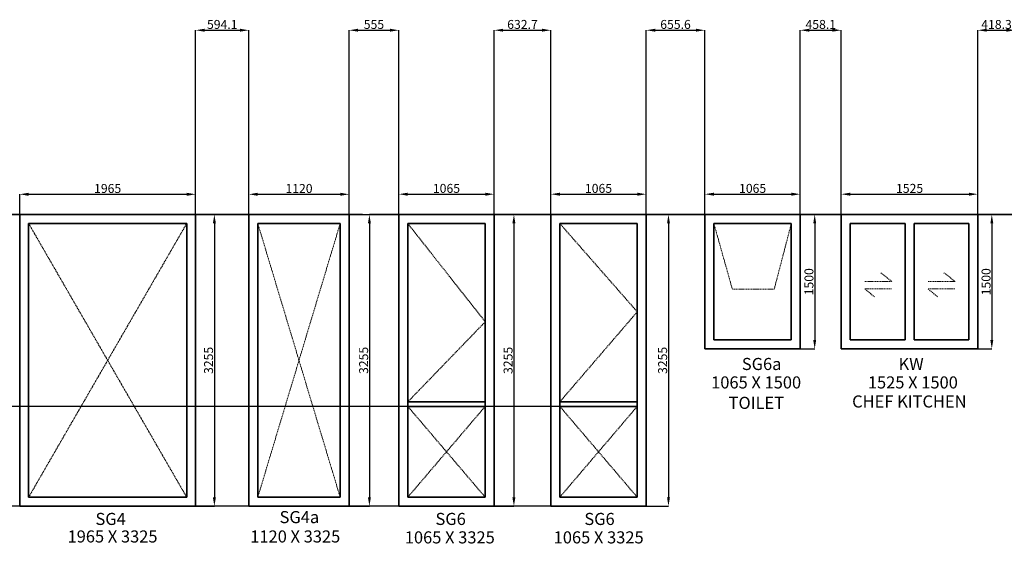
# Model space of a CAD drawing. Units: millimetres. Extents: x -850 to 42148, y -7352 to 4589.
# Tile 3 of 4: x 11314 to 22310, y -1278 to 4589. Entities that reach past the tile are written whole.
import ezdxf

# ---------------------------------------------------------------- set-up
doc = ezdxf.new("R2010")
doc.units = ezdxf.units.MM
doc.linetypes.add('DASHED', pattern=[19.05, 12.7, -6.35])
for name, color, linetype, lineweight in [('A-ANNO-DIMS', 2, 'Continuous', 18), ('A-ANNO-TEXT', 7, 'Continuous', 18), ('A-GLAZ', 4, 'Continuous', 35), ('A-GLAZ-OPNG', 4, 'DASHED', 18)]:
    doc.layers.add(name, color=color, linetype=linetype, lineweight=lineweight)
doc.styles.get("Standard").update_dxf_attribs({"font": 'arial.ttf'})
doc.dimstyles.new('ISO-25', dxfattribs={"dimtxt": 100, "dimasz": 100, "dimexe": 1.25, "dimexo": 0.625, "dimtad": 1, "dimtxsty": 'Standard', "dimcen": 2.5, "dimadec": 0, "dimazin": 0, "dimtfac": 1, "dimtmove": 0, "dimatfit": 3, "dimfxl": 1, "dimarcsym": 0})

# ---------------------------------------------------------------- blocks, each defined once
blk = doc.blocks.new('*D7')
at = {"layer": 'A-ANNO-DIMS', "color": 0, "lineweight": -2, "transparency": 16777216}
for p, q in [((11314, 2415), (11314, 2641)), ((11414, 2640), (13179, 2640)), ((13279, 2415), (13279, 2641))]:
    blk.add_line(p, q, dxfattribs=at)
at = {"layer": 'A-ANNO-DIMS', "color": 0, "lineweight": 30, "transparency": 16777216}
for points in [[(11414, 2657), (11414, 2623), (11314, 2640)], [(13179, 2657), (13179, 2623), (13279, 2640)]]:
    blk.add_solid(points, dxfattribs=at)
at = {"layer": 'Defpoints', "color": 0, "lineweight": 30, "transparency": 16777216}
for p in [(13279, 2640), (11314, 2414), (13279, 2414)]:
    blk.add_point(p, dxfattribs=at)
at = {"layer": 'A-ANNO-DIMS', "color": 0, "transparency": 16777216, "insert": (12296, 2692), "char_height": 100, "attachment_point": 5}
blk.add_mtext('1965', dxfattribs=at)
blk = doc.blocks.new('*D8')
at = {"layer": 'A-ANNO-DIMS', "color": 0, "lineweight": -2, "transparency": 16777216}
for p, q in [((13279, 2414), (13489, 2414)), ((13488, 2314), (13488, -741)), ((13279, -841), (13489, -841))]:
    blk.add_line(p, q, dxfattribs=at)
at = {"layer": 'A-ANNO-DIMS', "color": 0, "lineweight": 30, "transparency": 16777216}
for points in [[(13471, 2314), (13505, 2314), (13488, 2414)], [(13471, -741), (13505, -741), (13488, -841)]]:
    blk.add_solid(points, dxfattribs=at)
at = {"layer": 'Defpoints', "color": 0, "lineweight": 30, "transparency": 16777216}
for p in [(13279, 2414), (13279, -841), (13488, -841)]:
    blk.add_point(p, dxfattribs=at)
at = {"layer": 'A-ANNO-DIMS', "color": 0, "transparency": 16777216, "insert": (13436, 786), "char_height": 100, "attachment_point": 5, "rotation": 90}
blk.add_mtext('3255', dxfattribs=at)
blk = doc.blocks.new('*D9')
at = {"layer": 'A-ANNO-DIMS', "color": 0, "lineweight": -2, "transparency": 16777216}
for p, q in [((13873, 2415), (13873, 2641)), ((13973, 2640), (14893, 2640)), ((14993, 2415), (14993, 2641))]:
    blk.add_line(p, q, dxfattribs=at)
at = {"layer": 'A-ANNO-DIMS', "color": 0, "lineweight": 30, "transparency": 16777216}
for points in [[(13973, 2657), (13973, 2623), (13873, 2640)], [(14893, 2657), (14893, 2623), (14993, 2640)]]:
    blk.add_solid(points, dxfattribs=at)
at = {"layer": 'Defpoints', "color": 0, "lineweight": 30, "transparency": 16777216}
for p in [(14993, 2640), (13873, 2414), (14993, 2414)]:
    blk.add_point(p, dxfattribs=at)
at = {"layer": 'A-ANNO-DIMS', "color": 0, "transparency": 16777216, "insert": (14433, 2692), "char_height": 100, "attachment_point": 5}
blk.add_mtext('1120', dxfattribs=at)
blk = doc.blocks.new('*D10')
at = {"layer": 'A-ANNO-DIMS', "color": 0, "lineweight": -2, "transparency": 16777216}
for p, q in [((14994, 2414), (15221, 2414)), ((15219, 2314), (15219, -741)), ((14994, -841), (15221, -841))]:
    blk.add_line(p, q, dxfattribs=at)
at = {"layer": 'A-ANNO-DIMS', "color": 0, "lineweight": 30, "transparency": 16777216}
for points in [[(15203, 2314), (15236, 2314), (15219, 2414)], [(15203, -741), (15236, -741), (15219, -841)]]:
    blk.add_solid(points, dxfattribs=at)
at = {"layer": 'Defpoints', "color": 0, "lineweight": 30, "transparency": 16777216}
for p in [(14993, 2414), (14993, -841), (15219, -841)]:
    blk.add_point(p, dxfattribs=at)
at = {"layer": 'A-ANNO-DIMS', "color": 0, "transparency": 16777216, "insert": (15168, 786), "char_height": 100, "attachment_point": 5, "rotation": 90}
blk.add_mtext('3255', dxfattribs=at)
blk = doc.blocks.new('*D11')
at = {"layer": 'A-ANNO-DIMS', "color": 0, "lineweight": -2, "transparency": 16777216}
for p, q in [((15548, 2415), (15548, 2642)), ((15648, 2641), (16513, 2641)), ((16613, 2415), (16613, 2642))]:
    blk.add_line(p, q, dxfattribs=at)
at = {"layer": 'A-ANNO-DIMS', "color": 0, "lineweight": 30, "transparency": 16777216}
for points in [[(15648, 2658), (15648, 2624), (15548, 2641)], [(16513, 2658), (16513, 2624), (16613, 2641)]]:
    blk.add_solid(points, dxfattribs=at)
at = {"layer": 'Defpoints', "color": 0, "lineweight": 30, "transparency": 16777216}
for p in [(16613, 2641), (15548, 2414), (16613, 2414)]:
    blk.add_point(p, dxfattribs=at)
at = {"layer": 'A-ANNO-DIMS', "color": 0, "transparency": 16777216, "insert": (16080, 2693), "char_height": 100, "attachment_point": 5}
blk.add_mtext('1065', dxfattribs=at)
blk = doc.blocks.new('*D12')
at = {"layer": 'A-ANNO-DIMS', "color": 0, "lineweight": -2, "transparency": 16777216}
for p, q in [((16614, 2414), (16834, 2414)), ((16833, 2314), (16833, -741)), ((16614, -841), (16834, -841))]:
    blk.add_line(p, q, dxfattribs=at)
at = {"layer": 'A-ANNO-DIMS', "color": 0, "lineweight": 30, "transparency": 16777216}
for points in [[(16816, 2314), (16850, 2314), (16833, 2414)], [(16816, -741), (16850, -741), (16833, -841)]]:
    blk.add_solid(points, dxfattribs=at)
at = {"layer": 'Defpoints', "color": 0, "lineweight": 30, "transparency": 16777216}
for p in [(16613, 2414), (16613, -841), (16833, -841)]:
    blk.add_point(p, dxfattribs=at)
at = {"layer": 'A-ANNO-DIMS', "color": 0, "transparency": 16777216, "insert": (16781, 786), "char_height": 100, "attachment_point": 5, "rotation": 90}
blk.add_mtext('3255', dxfattribs=at)
blk = doc.blocks.new('*D13')
at = {"layer": 'A-ANNO-DIMS', "color": 0, "lineweight": -2, "transparency": 16777216}
for p, q in [((17246, 2415), (17246, 2642)), ((17346, 2641), (18211, 2641)), ((18311, 2415), (18311, 2642))]:
    blk.add_line(p, q, dxfattribs=at)
at = {"layer": 'A-ANNO-DIMS', "color": 0, "lineweight": 30, "transparency": 16777216}
for points in [[(17346, 2658), (17346, 2624), (17246, 2641)], [(18211, 2658), (18211, 2624), (18311, 2641)]]:
    blk.add_solid(points, dxfattribs=at)
at = {"layer": 'Defpoints', "color": 0, "lineweight": 30, "transparency": 16777216}
for p in [(18311, 2641), (17246, 2414), (18311, 2414)]:
    blk.add_point(p, dxfattribs=at)
at = {"layer": 'A-ANNO-DIMS', "color": 0, "transparency": 16777216, "insert": (17778, 2693), "char_height": 100, "attachment_point": 5}
blk.add_mtext('1065', dxfattribs=at)
blk = doc.blocks.new('*D14')
at = {"layer": 'A-ANNO-DIMS', "color": 0, "lineweight": -2, "transparency": 16777216}
for p, q in [((18311, 2414), (18560, 2414)), ((18559, 2314), (18559, -741)), ((18311, -841), (18560, -841))]:
    blk.add_line(p, q, dxfattribs=at)
at = {"layer": 'A-ANNO-DIMS', "color": 0, "lineweight": 30, "transparency": 16777216}
for points in [[(18543, 2314), (18576, 2314), (18559, 2414)], [(18543, -741), (18576, -741), (18559, -841)]]:
    blk.add_solid(points, dxfattribs=at)
at = {"layer": 'Defpoints', "color": 0, "lineweight": 30, "transparency": 16777216}
for p in [(18311, 2414), (18311, -841), (18559, -841)]:
    blk.add_point(p, dxfattribs=at)
at = {"layer": 'A-ANNO-DIMS', "color": 0, "transparency": 16777216, "insert": (18507, 786), "char_height": 100, "attachment_point": 5, "rotation": 90}
blk.add_mtext('3255', dxfattribs=at)
blk = doc.blocks.new('*D15')
at = {"layer": 'A-ANNO-DIMS', "color": 0, "lineweight": -2, "transparency": 16777216}
for p, q in [((18966, 2415), (18966, 2642)), ((19066, 2641), (19931, 2641)), ((20031, 2415), (20031, 2642))]:
    blk.add_line(p, q, dxfattribs=at)
at = {"layer": 'A-ANNO-DIMS', "color": 0, "lineweight": 30, "transparency": 16777216}
for points in [[(19066, 2658), (19066, 2624), (18966, 2641)], [(19931, 2658), (19931, 2624), (20031, 2641)]]:
    blk.add_solid(points, dxfattribs=at)
at = {"layer": 'Defpoints', "color": 0, "lineweight": 30, "transparency": 16777216}
for p in [(20031, 2641), (18966, 2414), (20031, 2414)]:
    blk.add_point(p, dxfattribs=at)
at = {"layer": 'A-ANNO-DIMS', "color": 0, "transparency": 16777216, "insert": (19499, 2693), "char_height": 100, "attachment_point": 5}
blk.add_mtext('1065', dxfattribs=at)
blk = doc.blocks.new('*D16')
at = {"layer": 'A-ANNO-DIMS', "color": 0, "lineweight": -2, "transparency": 16777216}
for p, q in [((20032, 2414), (20194, 2414)), ((20192, 2314), (20192, 1014)), ((20032, 914), (20194, 914))]:
    blk.add_line(p, q, dxfattribs=at)
at = {"layer": 'A-ANNO-DIMS', "color": 0, "lineweight": 30, "transparency": 16777216}
for points in [[(20176, 2314), (20209, 2314), (20192, 2414)], [(20176, 1014), (20209, 1014), (20192, 914)]]:
    blk.add_solid(points, dxfattribs=at)
at = {"layer": 'Defpoints', "color": 0, "lineweight": 30, "transparency": 16777216}
for p in [(20031, 2414), (20031, 914), (20192, 914)]:
    blk.add_point(p, dxfattribs=at)
at = {"layer": 'A-ANNO-DIMS', "color": 0, "transparency": 16777216, "insert": (20141, 1664), "char_height": 100, "attachment_point": 5, "rotation": 90}
blk.add_mtext('1500', dxfattribs=at)
blk = doc.blocks.new('*D17')
at = {"layer": 'A-ANNO-DIMS', "color": 0, "lineweight": -2, "transparency": 16777216}
for p, q in [((20489, 2415), (20489, 2642)), ((20589, 2641), (21914, 2641)), ((22014, 2415), (22014, 2642))]:
    blk.add_line(p, q, dxfattribs=at)
at = {"layer": 'A-ANNO-DIMS', "color": 0, "lineweight": 30, "transparency": 16777216}
for points in [[(20589, 2658), (20589, 2624), (20489, 2641)], [(21914, 2658), (21914, 2624), (22014, 2641)]]:
    blk.add_solid(points, dxfattribs=at)
at = {"layer": 'Defpoints', "color": 0, "lineweight": 30, "transparency": 16777216}
for p in [(22014, 2641), (20489, 2414), (22014, 2414)]:
    blk.add_point(p, dxfattribs=at)
at = {"layer": 'A-ANNO-DIMS', "color": 0, "transparency": 16777216, "insert": (21252, 2693), "char_height": 100, "attachment_point": 5}
blk.add_mtext('1525', dxfattribs=at)
blk = doc.blocks.new('*D18')
at = {"layer": 'A-ANNO-DIMS', "color": 0, "lineweight": -2, "transparency": 16777216}
for p, q in [((22015, 2414), (22172, 2414)), ((22170, 2314), (22170, 1014)), ((22015, 914), (22172, 914))]:
    blk.add_line(p, q, dxfattribs=at)
at = {"layer": 'A-ANNO-DIMS', "color": 0, "lineweight": 30, "transparency": 16777216}
for points in [[(22154, 2314), (22187, 2314), (22170, 2414)], [(22154, 1014), (22187, 1014), (22170, 914)]]:
    blk.add_solid(points, dxfattribs=at)
at = {"layer": 'Defpoints', "color": 0, "lineweight": 30, "transparency": 16777216}
for p in [(22014, 2414), (22014, 914), (22170, 914)]:
    blk.add_point(p, dxfattribs=at)
at = {"layer": 'A-ANNO-DIMS', "color": 0, "transparency": 16777216, "insert": (22119, 1664), "char_height": 100, "attachment_point": 5, "rotation": 90}
blk.add_mtext('1500', dxfattribs=at)
blk = doc.blocks.new('*D60')
at = {"layer": 'A-ANNO-DIMS', "color": 0, "lineweight": -2, "transparency": 16777216}
for p, q in [((41489, -432), (41489, -2900)), ((1325, -812), (1325, -2900)), ((1425, -2899), (41389, -2899))]:
    blk.add_line(p, q, dxfattribs=at)
at = {"layer": 'A-ANNO-DIMS', "color": 0, "lineweight": 30, "transparency": 16777216}
for points in [[(1425, -2882), (1425, -2915), (1325, -2899)], [(41389, -2882), (41389, -2915), (41489, -2899)]]:
    blk.add_solid(points, dxfattribs=at)
at = {"layer": 'Defpoints', "color": 0, "lineweight": 30, "transparency": 16777216}
for p in [(41489, -431), (1325, -811), (41489, -2899)]:
    blk.add_point(p, dxfattribs=at)
at = {"layer": 'A-ANNO-DIMS', "color": 0, "transparency": 16777216, "insert": (21407, -2847), "char_height": 100, "attachment_point": 5}
blk.add_mtext('40164', dxfattribs=at)
blk = doc.blocks.new('*D64')
at = {"layer": 'A-ANNO-DIMS', "color": 0, "lineweight": -2, "transparency": 16777216}
for p, q in [((13279, 2415), (13279, 4473)), ((13379, 4471), (13773, 4471)), ((13873, 2415), (13873, 4473))]:
    blk.add_line(p, q, dxfattribs=at)
at = {"layer": 'A-ANNO-DIMS', "color": 0, "lineweight": 30, "transparency": 16777216}
for points in [[(13379, 4488), (13379, 4455), (13279, 4471)], [(13773, 4488), (13773, 4455), (13873, 4471)]]:
    blk.add_solid(points, dxfattribs=at)
at = {"layer": 'Defpoints', "color": 0, "lineweight": 30, "transparency": 16777216}
for p in [(13873, 4471), (13279, 2414), (13873, 2414)]:
    blk.add_point(p, dxfattribs=at)
at = {"layer": 'A-ANNO-DIMS', "color": 0, "transparency": 16777216, "insert": (13576, 4523), "char_height": 100, "attachment_point": 5}
blk.add_mtext('594.1', dxfattribs=at)
blk = doc.blocks.new('*D65')
at = {"layer": 'A-ANNO-DIMS', "color": 0, "lineweight": -2, "transparency": 16777216}
for p, q in [((14993, 2415), (14993, 4473)), ((15093, 4471), (15448, 4471)), ((15548, 2415), (15548, 4473))]:
    blk.add_line(p, q, dxfattribs=at)
at = {"layer": 'A-ANNO-DIMS', "color": 0, "lineweight": 30, "transparency": 16777216}
for points in [[(15093, 4488), (15093, 4455), (14993, 4471)], [(15448, 4488), (15448, 4455), (15548, 4471)]]:
    blk.add_solid(points, dxfattribs=at)
at = {"layer": 'Defpoints', "color": 0, "lineweight": 30, "transparency": 16777216}
for p in [(15548, 4471), (14993, 2414), (15548, 2414)]:
    blk.add_point(p, dxfattribs=at)
at = {"layer": 'A-ANNO-DIMS', "color": 0, "transparency": 16777216, "insert": (15270, 4523), "char_height": 100, "attachment_point": 5}
blk.add_mtext('555', dxfattribs=at)
blk = doc.blocks.new('*D66')
at = {"layer": 'A-ANNO-DIMS', "color": 0, "lineweight": -2, "transparency": 16777216}
for p, q in [((16613, 2415), (16613, 4473)), ((16713, 4471), (17146, 4471)), ((17246, 2415), (17246, 4473))]:
    blk.add_line(p, q, dxfattribs=at)
at = {"layer": 'A-ANNO-DIMS', "color": 0, "lineweight": 30, "transparency": 16777216}
for points in [[(16713, 4488), (16713, 4455), (16613, 4471)], [(17146, 4488), (17146, 4455), (17246, 4471)]]:
    blk.add_solid(points, dxfattribs=at)
at = {"layer": 'Defpoints', "color": 0, "lineweight": 30, "transparency": 16777216}
for p in [(17246, 4471), (16613, 2414), (17246, 2414)]:
    blk.add_point(p, dxfattribs=at)
at = {"layer": 'A-ANNO-DIMS', "color": 0, "transparency": 16777216, "insert": (16929, 4523), "char_height": 100, "attachment_point": 5}
blk.add_mtext('632.7', dxfattribs=at)
blk = doc.blocks.new('*D67')
at = {"layer": 'A-ANNO-DIMS', "color": 0, "lineweight": -2, "transparency": 16777216}
for p, q in [((18311, 2415), (18311, 4473)), ((18411, 4471), (18866, 4471)), ((18966, 2415), (18966, 4473))]:
    blk.add_line(p, q, dxfattribs=at)
at = {"layer": 'A-ANNO-DIMS', "color": 0, "lineweight": 30, "transparency": 16777216}
for points in [[(18411, 4488), (18411, 4455), (18311, 4471)], [(18866, 4488), (18866, 4455), (18966, 4471)]]:
    blk.add_solid(points, dxfattribs=at)
at = {"layer": 'Defpoints', "color": 0, "lineweight": 30, "transparency": 16777216}
for p in [(18966, 4471), (18311, 2414), (18966, 2414)]:
    blk.add_point(p, dxfattribs=at)
at = {"layer": 'A-ANNO-DIMS', "color": 0, "transparency": 16777216, "insert": (18638, 4523), "char_height": 100, "attachment_point": 5}
blk.add_mtext('655.6', dxfattribs=at)
blk = doc.blocks.new('*D68')
at = {"layer": 'A-ANNO-DIMS', "color": 0, "lineweight": -2, "transparency": 16777216}
for p, q in [((20031, 2415), (20031, 4473)), ((20131, 4471), (20389, 4471)), ((20489, 2415), (20489, 4473))]:
    blk.add_line(p, q, dxfattribs=at)
at = {"layer": 'A-ANNO-DIMS', "color": 0, "lineweight": 30, "transparency": 16777216}
for points in [[(20131, 4488), (20131, 4455), (20031, 4471)], [(20389, 4488), (20389, 4455), (20489, 4471)]]:
    blk.add_solid(points, dxfattribs=at)
at = {"layer": 'Defpoints', "color": 0, "lineweight": 30, "transparency": 16777216}
for p in [(20489, 4471), (20031, 2414), (20489, 2414)]:
    blk.add_point(p, dxfattribs=at)
at = {"layer": 'A-ANNO-DIMS', "color": 0, "transparency": 16777216, "insert": (20260, 4523), "char_height": 100, "attachment_point": 5}
blk.add_mtext('458.1', dxfattribs=at)
blk = doc.blocks.new('*D69')
at = {"layer": 'A-ANNO-DIMS', "color": 0, "lineweight": -2, "transparency": 16777216}
for p, q in [((22014, 2415), (22014, 4473)), ((22114, 4471), (22333, 4471)), ((22433, 2415), (22433, 4473))]:
    blk.add_line(p, q, dxfattribs=at)
at = {"layer": 'A-ANNO-DIMS', "color": 0, "lineweight": 30, "transparency": 16777216}
for points in [[(22114, 4488), (22114, 4455), (22014, 4471)], [(22333, 4488), (22333, 4455), (22433, 4471)]]:
    blk.add_solid(points, dxfattribs=at)
at = {"layer": 'Defpoints', "color": 0, "lineweight": 30, "transparency": 16777216}
for p in [(22433, 4471), (22014, 2414), (22433, 2414)]:
    blk.add_point(p, dxfattribs=at)
at = {"layer": 'A-ANNO-DIMS', "color": 0, "transparency": 16777216, "insert": (22223, 4523), "char_height": 100, "attachment_point": 5}
blk.add_mtext('418.3', dxfattribs=at)
blk = doc.blocks.new('*D74')
at = {"layer": 'A-ANNO-DIMS', "color": 0, "lineweight": -2, "transparency": 16777216}
for p, q in [((17345, 273), (-734, 273)), ((-732, -741), (-732, 173)), ((17245, -841), (-734, -841))]:
    blk.add_line(p, q, dxfattribs=at)
at = {"layer": 'A-ANNO-DIMS', "color": 0, "lineweight": 30, "transparency": 16777216}
for points in [[(-749, 173), (-716, 173), (-732, 273)], [(-749, -741), (-716, -741), (-732, -841)]]:
    blk.add_solid(points, dxfattribs=at)
at = {"layer": 'Defpoints', "color": 0, "lineweight": 30, "transparency": 16777216}
for p in [(-732, 273), (17346, 273), (17246, -841)]:
    blk.add_point(p, dxfattribs=at)
at = {"layer": 'A-ANNO-DIMS', "color": 0, "transparency": 16777216, "insert": (-784, -284), "char_height": 100, "attachment_point": 5, "rotation": 90}
blk.add_mtext('1113.8', dxfattribs=at)

msp = doc.modelspace()

# ---------------------------------------------------------------- linework, layer by layer
at = {"layer": 'A-GLAZ'}
for p, q in [((1325.061, 2413.876), (15141.402, 2413.876)), ((11313.76, 2413.876), (11313.76, -841.124)), ((11413.76, 2313.876), (11413.76, -741.124)), ((11413.76, 2313.876), (13178.76, 2313.876)), ((13178.76, -741.124), (13178.76, 2313.876)), ((13278.76, -841.124), (13278.76, 2413.876)), ((13872.899, 2413.876), (13872.899, -841.124)), ((13972.899, 2313.876), (13972.899, -741.124)), ((13972.899, 2313.876), (14892.899, 2313.876)), ((14892.899, -741.124), (14892.899, 2313.876)), ((14992.899, -841.124), (14992.899, 2413.876)), ((15219.457, 2413.876), (42147.613, 2413.876)), ((15547.901, 2413.876), (15547.901, -841.124)), ((15647.901, 2313.876), (15647.901, -741.124)), ((15647.901, 2313.876), (16512.901, 2313.876)), ((16512.901, -741.124), (16512.901, 2313.876)), ((16612.901, -841.124), (16612.901, 2413.876)), ((17245.641, 2413.876), (17245.641, -841.124)), ((17345.641, 2313.876), (18210.641, 2313.876)), ((17345.641, 2313.876), (17345.641, -741.124)), ((18210.641, -741.124), (18210.641, 2313.876)), ((18310.641, -841.124), (18310.641, 2413.876)), ((18966.202, 2413.876), (18966.202, 913.876)), ((19066.202, 2313.876), (19931.202, 2313.876)), ((19066.202, 2313.876), (19066.202, 1013.876)), ((19931.202, 1013.876), (19931.202, 2313.876)), ((20031.202, 913.876), (20031.202, 2413.876)), ((20489.328, 2413.876), (20489.328, 913.876)), ((20589.328, 2313.876), (20589.328, 1013.876)), ((20589.328, 2313.876), (21201.828, 2313.876)), ((21201.828, 1013.876), (21201.828, 2313.876)), ((21301.828, 1013.876), (21301.828, 2313.876)), ((21301.828, 2313.876), (21914.328, 2313.876)), ((21914.328, 1013.876), (21914.328, 2313.876)), ((22014.328, 913.876), (22014.328, 2413.876)), ((19066.202, 1013.876), (19931.202, 1013.876)), ((20589.328, 1013.876), (21201.828, 1013.876)), ((21301.828, 1013.876), (21914.328, 1013.876)), ((18966.202, 913.876), (20031.202, 913.876)), ((20489.328, 913.876), (22014.328, 913.876)), ((15647.901, 322.698), (16512.901, 322.698)), ((15647.901, 272.698), (16512.901, 272.698)), ((17345.641, 322.698), (18210.641, 322.698)), ((17345.641, 272.698), (18210.641, 272.698)), ((11413.76, -741.124), (13178.76, -741.124)), ((13972.899, -741.124), (14892.899, -741.124)), ((15647.901, -741.124), (16512.901, -741.124)), ((17345.641, -741.124), (18210.641, -741.124)), ((11313.76, -841.124), (13278.76, -841.124)), ((13872.899, -841.124), (14992.899, -841.124)), ((15547.901, -841.124), (16612.901, -841.124)), ((17245.641, -841.124), (18310.641, -841.124))]:
    msp.add_line(p, q, dxfattribs=at)
at = {"layer": 'A-GLAZ-OPNG'}
for p, q in [((11413.76, 2313.876), (13178.76, -741.124)), ((11413.76, -741.124), (13178.76, 2313.876)), ((13972.899, 2313.876), (14892.899, -741.124)), ((13972.899, -741.124), (14892.899, 2313.876)), ((15647.901, 2313.876), (16512.901, 1216.635)), ((17345.641, 2313.876), (18210.641, 1328.216)), ((19066.202, 2313.876), (19273.187, 1579.849)), ((19931.202, 2313.876), (19740.078, 1579.849)), ((21055.084, 1667.266), (20929.637, 1762.912)), ((21761.05, 1667.266), (21635.603, 1762.912)), ((20752.085, 1667.266), (21055.084, 1667.266)), ((21458.051, 1667.266), (21761.05, 1667.266)), ((19273.187, 1579.849), (19740.078, 1579.849)), ((20752.988, 1583.878), (21055.987, 1583.878)), ((20752.988, 1583.878), (20860.514, 1494.362)), ((21458.953, 1583.878), (21761.952, 1583.878)), ((21458.953, 1583.878), (21566.479, 1494.362)), ((18210.641, 1328.216), (17345.641, 322.698)), ((16512.901, 1216.635), (15647.901, 322.698)), ((15647.901, 272.698), (16512.901, -741.124)), ((16512.901, 272.698), (15647.901, -741.124)), ((17345.641, 272.698), (18210.641, -741.124)), ((18210.641, 272.698), (17345.641, -741.124))]:
    msp.add_line(p, q, dxfattribs=at)

# ---------------------------------------------------------------- texts
at = {"layer": 'A-ANNO-TEXT'}
for s, height, p in [('SG6a', 134.8889, (19378.659, 678.488)), ('KW', 134.8889, (21128.786, 678.488)), ('1065 X 1500', 134.88886, (19035.885, 472.651)), ('1525 X 1500', 134.88886, (20786.012, 472.651)), ('TOILET', 134.8889, (19230.903, 244.607)), ('CHEF KITCHEN', 134.88886, (20610.253, 260.041)), ('SG4', 134.8889, (12160.079, -1051.132)), ('SG4a', 134.8889, (14216.2, -1030.64)), ('SG6', 134.8889, (15957.341, -1051.132)), ('SG6', 134.8889, (17619.962, -1051.132)), ('1965 X 3325', 134.88886, (11848.074, -1246.723)), ('1120 X 3325', 134.88886, (13888.81, -1246.723)), ('1065 X 3325', 134.88886, (15614.568, -1256.969)), ('1065 X 3325', 134.88886, (17277.188, -1256.969))]:
    msp.add_text(s, height=height, dxfattribs=at).set_placement(p)

# ---------------------------------------------------------------- dimensions: what is measured, and where the dimension line sits
at = {"layer": 'A-ANNO-DIMS'}
for base, p1, p2, override, picture, middle in [((13872.899, 4471.376), (13278.76, 2413.876), (13872.899, 2413.876), {"dimdec": 1, "dimlfac": 1, "dimrnd": 0, "dimzin": 0, "dimdsep": 46, "dimlunit": 2}, '*D64', (13575.829, 4523.058)), ((15547.901, 4471.376), (14992.899, 2413.876), (15547.901, 2413.876), {"dimdec": 0, "dimlfac": 1, "dimrnd": 0, "dimzin": 0, "dimdsep": 46, "dimlunit": 2}, '*D65', (15270.4, 4522.854)), ((17245.641, 4471.376), (16612.901, 2413.876), (17245.641, 2413.876), {"dimdec": 1, "dimlfac": 1, "dimrnd": 0, "dimzin": 0, "dimdsep": 46, "dimlunit": 2}, '*D66', (16929.271, 4523.092)), ((18966.202, 4471.376), (18310.641, 2413.876), (18966.202, 2413.876), {"dimdec": 1, "dimlfac": 1, "dimrnd": 0, "dimzin": 0, "dimdsep": 46, "dimlunit": 2}, '*D67', (18638.422, 4523.058)), ((20489.328, 4471.376), (20031.202, 2413.876), (20489.328, 2413.876), {"dimdec": 1, "dimlfac": 1, "dimrnd": 0, "dimzin": 0, "dimdsep": 46, "dimlunit": 2}, '*D68', (20260.265, 4523.058)), ((22432.638, 4471.376), (22014.328, 2413.876), (22432.638, 2413.876), {"dimdec": 1, "dimlfac": 1, "dimrnd": 0, "dimzin": 0, "dimdsep": 46, "dimlunit": 2}, '*D69', (22223.483, 4523.092)), ((13278.76, 2639.846), (11313.76, 2413.876), (13278.76, 2413.876), {"dimclrd": 0, "dimclre": 0, "dimclrt": 0}, '*D7', (12296.26, 2691.528)), ((14992.899, 2639.846), (13872.899, 2413.876), (14992.899, 2413.876), {"dimclrd": 0, "dimclre": 0, "dimclrt": 0}, '*D9', (14432.899, 2691.528)), ((16612.901, 2641.096), (15547.901, 2413.876), (16612.901, 2413.876), {"dimclrd": 0, "dimclre": 0, "dimclrt": 0}, '*D11', (16080.401, 2692.778)), ((18310.641, 2641.096), (17245.641, 2413.876), (18310.641, 2413.876), {"dimclrd": 0, "dimclre": 0, "dimclrt": 0}, '*D13', (17778.141, 2692.778)), ((20031.202, 2641.096), (18966.202, 2413.876), (20031.202, 2413.876), {"dimclrd": 0, "dimclre": 0, "dimclrt": 0}, '*D15', (19498.702, 2692.778)), ((22014.328, 2641.096), (20489.328, 2413.876), (22014.328, 2413.876), {"dimclrd": 0, "dimclre": 0, "dimclrt": 0}, '*D17', (21251.828, 2692.778)), ((41488.766, -2898.624), (1325.061, -811.124), (41488.766, -431.124), {"dimdec": 0, "dimlfac": 1, "dimrnd": 0, "dimzin": 0, "dimdsep": 46, "dimlunit": 2}, '*D60', (21406.913, -2846.942))]:
    dim = msp.add_linear_dim(base=base, p1=p1, p2=p2, dimstyle='ISO-25', override=override, dxfattribs=at)
    dim.commit()
    dim.dimension.update_dxf_attribs({"geometry": picture, "text_midpoint": middle})
for base, p1, p2, override, picture, middle in [((13488.009, -841.124), (13278.76, 2413.876), (13278.76, -841.124), {"dimclrd": 0, "dimclre": 0, "dimclrt": 0}, '*D8', (13436.293, 786.376)), ((15219.457, -841.124), (14992.899, 2413.876), (14992.899, -841.124), {"dimclrd": 0, "dimclre": 0, "dimclrt": 0}, '*D10', (15167.741, 786.376)), ((16833.059, -841.124), (16612.901, 2413.876), (16612.901, -841.124), {"dimclrd": 0, "dimclre": 0, "dimclrt": 0}, '*D12', (16781.343, 786.376)), ((18559.195, -841.124), (18310.641, 2413.876), (18310.641, -841.124), {"dimclrd": 0, "dimclre": 0, "dimclrt": 0}, '*D14', (18507.479, 786.376)), ((20192.294, 913.876), (20031.202, 2413.876), (20031.202, 913.876), {"dimclrd": 0, "dimclre": 0, "dimclrt": 0}, '*D16', (20140.612, 1663.876)), ((22170.352, 913.876), (22014.328, 2413.876), (22014.328, 913.876), {"dimclrd": 0, "dimclre": 0, "dimclrt": 0}, '*D18', (22118.669, 1663.876)), ((-732.439, 272.698), (17245.641, -841.124), (17345.641, 272.698), {"dimdec": 1, "dimlfac": 1, "dimrnd": 0, "dimzin": 0, "dimdsep": 46, "dimlunit": 2}, '*D74', (-784.156, -284.213))]:
    dim = msp.add_linear_dim(base=base, p1=p1, p2=p2, angle=90, dimstyle='ISO-25', override=override, dxfattribs=at)
    dim.commit()
    dim.dimension.update_dxf_attribs({"geometry": picture, "text_midpoint": middle})

doc.saveas('drawing.dxf')
